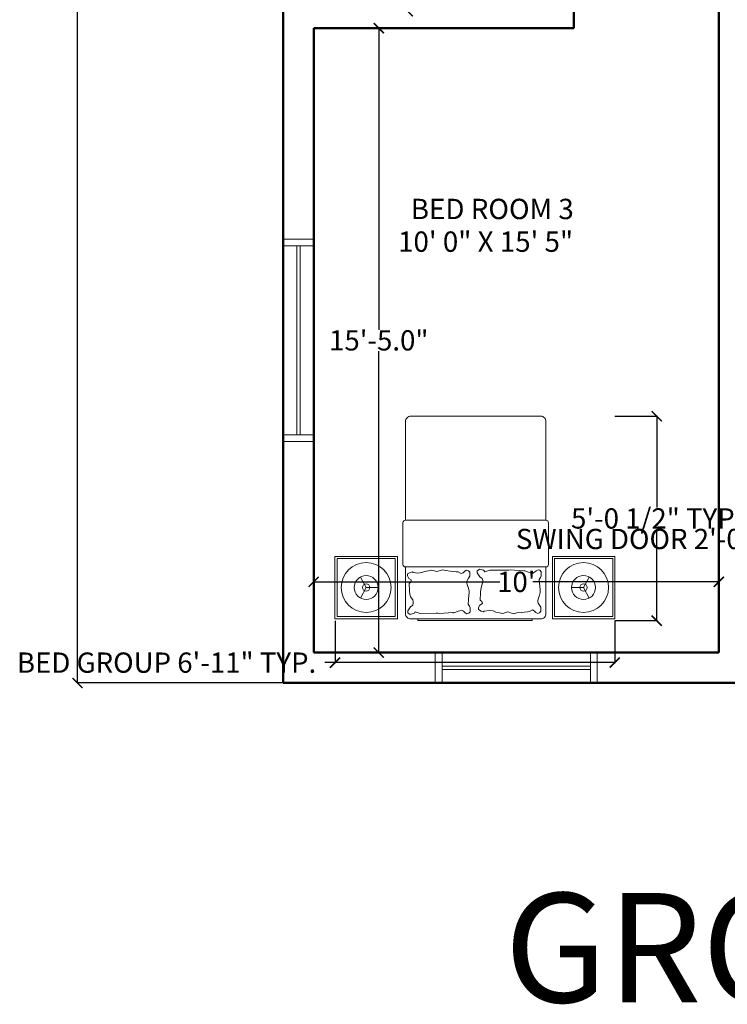
# Model space of a CAD drawing. Units: inches. Extents: x 147 to 1638, y 107 to 941.
# Tile 1 of 17: x 147 to 356, y 107 to 398. Entities that reach past the tile are written whole.
import ezdxf

# ---------------------------------------------------------------- set-up
doc = ezdxf.new("R2010")
doc.units = ezdxf.units.IN
doc.header["$MEASUREMENT"] = 0
for name, color, linetype, lineweight in [('A-ANNO-DIMS', 2, 'Continuous', 15), ('A-ANNO-TEXT', 7, 'Continuous', 25), ('A-AREA-IDEN', 7, 'Continuous', 18), ('furniture', 50, 'Continuous', 18), ('walls', 7, 'Continuous', 50), ('windows', 3, 'Continuous', 20)]:
    doc.layers.add(name, color=color, linetype=linetype, lineweight=lineweight)
doc.styles.get("Standard").update_dxf_attribs({"font": 'arial.ttf'})
doc.dimstyles.get("Standard").update_dxf_attribs({"dimtxt": 6, "dimasz": 3, "dimexe": 0.18, "dimexo": 0.0625, "dimgap": 0.09, "dimtad": 0, "dimtih": 1, "dimtoh": 1, "dimdec": 1, "dimzin": 0, "dimdsep": 46, "dimlunit": 3, "dimtxsty": 'Standard', "dimblk": 'ARCHTICK', "dimcen": 0.09, "dimadec": 0, "dimazin": 0, "dimtfac": 1, "dimtdec": 1, "dimtofl": 0, "dimtmove": 0, "dimatfit": 3, "dimfxl": 1, "dimtolj": 1, "dimtzin": 0, "dimarcsym": 0})

# ---------------------------------------------------------------- blocks, each defined once
blk = doc.blocks.new('_ArchTick')
at = {"color": 0, "linetype": 'ByBlock', "const_width": 0.15}
blk.add_lwpolyline([(-0.5, -0.5), (0.5, 0.5)], dxfattribs=at)
blk = doc.blocks.new('*D24')
at = {"layer": 'A-ANNO-DIMS', "color": 0, "lineweight": -2, "transparency": 16777216}
for p, q in [((248.22, 395.72), (253.39, 395.72)), ((253.21, 395.72), (253.21, 306.37)), ((253.21, 210.72), (253.21, 300.06)), ((248.22, 210.72), (253.39, 210.72))]:
    blk.add_line(p, q, dxfattribs=at)
at = {"layer": 'Defpoints', "color": 0, "lineweight": -2, "transparency": 16777216}
for p in [(248.16, 395.72), (248.16, 210.72), (253.21, 210.72)]:
    blk.add_point(p, dxfattribs=at)
at = {"layer": 'A-ANNO-DIMS', "color": 0, "lineweight": -2, "transparency": 16777216, "xscale": 3, "yscale": 3, "zscale": 3}
for p, rotation in [((253.21, 395.72), 90), ((253.21, 210.72), 270)]:
    blk.add_blockref('_ArchTick', p, dxfattribs=dict(at, rotation=rotation))
at = {"layer": 'A-ANNO-DIMS', "color": 0, "transparency": 16777216, "insert": (253.21, 303.22), "char_height": 6, "attachment_point": 5}
blk.add_mtext('\\A1;15\'-5.0"', dxfattribs=at)
blk = doc.blocks.new('*D25')
at = {"layer": 'A-ANNO-DIMS', "color": 0, "lineweight": -2, "transparency": 16777216}
for p, q in [((233.94, 245.59), (233.94, 231.49)), ((353.94, 245.59), (353.94, 231.49)), ((233.94, 231.67), (289.05, 231.67)), ((353.94, 231.67), (298.84, 231.67))]:
    blk.add_line(p, q, dxfattribs=at)
at = {"layer": 'Defpoints', "color": 0, "lineweight": -2, "transparency": 16777216}
for p in [(233.94, 245.65), (353.94, 245.65), (353.94, 231.67)]:
    blk.add_point(p, dxfattribs=at)
at = {"layer": 'A-ANNO-DIMS', "color": 0, "lineweight": -2, "transparency": 16777216, "xscale": 3, "yscale": 3, "zscale": 3, "rotation": 180}
blk.add_blockref('_ArchTick', (233.94, 231.67), dxfattribs=at)
at = {"layer": 'A-ANNO-DIMS', "color": 0, "lineweight": -2, "transparency": 16777216, "xscale": 3, "yscale": 3, "zscale": 3}
blk.add_blockref('_ArchTick', (353.94, 231.67), dxfattribs=at)
at = {"layer": 'A-ANNO-DIMS', "color": 0, "transparency": 16777216, "insert": (293.94, 231.67), "char_height": 6, "attachment_point": 5}
blk.add_mtext("\\A1;10'", dxfattribs=at)
blk = doc.blocks.new('*D70')
at = {"layer": 'A-ANNO-DIMS', "color": 0, "lineweight": -2, "transparency": 16777216}
for p, q in [((224.88, 909.72), (163.8, 909.72)), ((163.98, 909.72), (163.98, 558.87)), ((163.98, 201.72), (163.98, 552.56)), ((224.88, 201.72), (163.8, 201.72))]:
    blk.add_line(p, q, dxfattribs=at)
at = {"layer": 'Defpoints', "color": 0, "lineweight": -2, "transparency": 16777216}
for p in [(224.94, 909.72), (163.98, 201.72), (224.94, 201.72)]:
    blk.add_point(p, dxfattribs=at)
at = {"layer": 'A-ANNO-DIMS', "color": 0, "lineweight": -2, "transparency": 16777216, "xscale": 3, "yscale": 3, "zscale": 3}
for p, rotation in [((163.98, 909.72), 90), ((163.98, 201.72), 270)]:
    blk.add_blockref('_ArchTick', p, dxfattribs=dict(at, rotation=rotation))
at = {"layer": 'A-ANNO-DIMS', "color": 0, "transparency": 16777216, "insert": (163.98, 555.72), "char_height": 6, "attachment_point": 5}
blk.add_mtext("\\A1;59'", dxfattribs=at)
blk = doc.blocks.new('MAT-P14')
for p, q in [((-1.3369, 1.348), (-1.3369, 1.948)), ((-1.3369, 1.948), (-0.7369, 1.948)), ((-1.3169, 1.928), (-0.7569, 1.928)), ((-1.3169, 1.368), (-1.3169, 1.928)), ((-0.7569, 1.368), (-0.7569, 1.928)), ((-0.7369, 1.348), (-0.7369, 1.948)), ((0.625, 1.95), (-0.625, 1.95)), ((0.7534, 1.348), (0.7534, 1.948)), ((1.3534, 1.948), (0.7534, 1.948)), ((1.3334, 1.928), (0.7734, 1.928)), ((0.7734, 1.368), (0.7734, 1.928)), ((1.3334, 1.368), (1.3334, 1.928)), ((1.3534, 1.348), (1.3534, 1.948)), ((-1.0369, 1.648), (-1.0913, 1.7493)), ((1.0534, 1.648), (1.1078, 1.7493)), ((-1.0369, 1.648), (-1.0913, 1.5467)), ((-1.0369, 1.648), (-0.9219, 1.648)), ((1.0534, 1.648), (0.9384, 1.648)), ((1.0534, 1.648), (1.1078, 1.5467)), ((-1.3369, 1.348), (-0.7369, 1.348)), ((-1.3169, 1.368), (-0.7569, 1.368)), ((1.3534, 1.348), (0.7534, 1.348)), ((1.3334, 1.368), (0.7734, 1.368))]:
    blk.add_line(p, q)
for points in [[(-0.675, 1.45), (-0.675, 1.9, -0.414214), (-0.625, 1.95), (0.625, 1.95, -0.414214), (0.675, 1.9), (0.675, 1.45)], [(-0.675, 1, -0.414214), (-0.7, 1.025), (-0.7, 1.425, -0.414214), (-0.675, 1.45), (0.675, 1.45, -0.414214), (0.7, 1.425), (0.7, 1.025, -0.414214), (0.675, 1)], [(-0.625, 0, -0.414214), (-0.675, 0.05), (-0.675, 1), (0.675, 1), (0.675, 0.05, -0.414214), (0.625, 0)]]:
    blk.add_lwpolyline(points, format="xyb", close=True)
for points in [[(-0.6142, 1.8182), (-0.6262, 1.8377), (-0.6262, 1.8767), (-0.6142, 1.8914), (-0.5964, 1.8963), (-0.5785, 1.8865), (-0.563, 1.8719), (-0.5451, 1.8633), (-0.5157, 1.879), (-0.4966, 1.8816), (-0.4647, 1.8842), (-0.4393, 1.8868), (-0.3947, 1.892), (-0.3629, 1.8999), (-0.3094, 1.8823), (-0.2619, 1.8969), (-0.23, 1.8916), (-0.1918, 1.8838), (-0.1664, 1.8734), (-0.1282, 1.8682), (-0.0818, 1.8753), (-0.0758, 1.8802), (-0.052, 1.8753), (-0.0281, 1.8607), (-0.0281, 1.8412), (-0.0401, 1.8168), (-0.0639, 1.8022), (-0.0598, 1.781), (-0.0431, 1.7682), (-0.0463, 1.6973), (-0.0502, 1.6621), (-0.0561, 1.6397), (-0.0619, 1.6125), (-0.0678, 1.5965), (-0.0678, 1.5789), (-0.0631, 1.5599), (-0.0393, 1.5453), (-0.0147, 1.5053), (-0.0147, 1.4858), (-0.0385, 1.4711), (-0.0751, 1.4819), (-0.081, 1.4868), (-0.087, 1.4965), (-0.1344, 1.4812), (-0.3042, 1.4815), (-0.3178, 1.4815), (-0.3355, 1.4791), (-0.4636, 1.4878), (-0.4672, 1.4865), (-0.4732, 1.4863), (-0.5167, 1.5026), (-0.5299, 1.5053), (-0.5478, 1.5102), (-0.5656, 1.5015), (-0.5812, 1.4869), (-0.599, 1.4772), (-0.6169, 1.482), (-0.6288, 1.4967), (-0.6288, 1.5357), (-0.6229, 1.5503), (-0.611, 1.5698), (-0.6136, 1.6138), (-0.6149, 1.6269), (-0.6176, 1.6443), (-0.6189, 1.6595), (-0.6202, 1.6748), (-0.6202, 1.6955), (-0.6176, 1.7075), (-0.6136, 1.7227), (-0.6083, 1.7391), (-0.6043, 1.75), (-0.5976, 1.7707), (-0.5963, 1.7848), (-0.6003, 1.7979), (-0.6136, 1.8186)], [(0.0694, 1.5591), (0.0575, 1.5396), (0.0575, 1.5006), (0.0694, 1.4859), (0.0873, 1.481), (0.1052, 1.4908), (0.1207, 1.5054), (0.1386, 1.514), (0.168, 1.4983), (0.1871, 1.4957), (0.2189, 1.4931), (0.2444, 1.4905), (0.289, 1.4853), (0.3208, 1.4774), (0.3742, 1.495), (0.4218, 1.4804), (0.4536, 1.4857), (0.4918, 1.4935), (0.5173, 1.5039), (0.5555, 1.5091), (0.6019, 1.502), (0.6079, 1.4971), (0.6317, 1.502), (0.6555, 1.5166), (0.6555, 1.5361), (0.6436, 1.5605), (0.6198, 1.5751), (0.6239, 1.5963), (0.6405, 1.6091), (0.6373, 1.68), (0.6334, 1.7152), (0.6276, 1.7376), (0.6063, 1.7648), (0.6005, 1.7808), (0.6005, 1.7984), (0.6051, 1.8174), (0.6289, 1.832), (0.6536, 1.872), (0.6536, 1.8915), (0.6298, 1.9062), (0.5932, 1.8954), (0.5872, 1.8905), (0.5813, 1.8808), (0.5338, 1.8961), (0.3795, 1.8958), (0.3658, 1.8958), (0.3482, 1.8982), (0.2201, 1.8895), (0.2165, 1.8908), (0.2104, 1.891), (0.1669, 1.8747), (0.1538, 1.872), (0.1359, 1.8671), (0.118, 1.8758), (0.1025, 1.8904), (0.0846, 1.9001), (0.0667, 1.8953), (0.0548, 1.8806), (0.0548, 1.8416), (0.0608, 1.827), (0.0727, 1.8075), (0.0701, 1.7635), (0.0688, 1.7504), (0.0661, 1.733), (0.0648, 1.7178), (0.0634, 1.7025), (0.0634, 1.6818), (0.0661, 1.6698), (0.0701, 1.6546), (0.0754, 1.6382), (0.0794, 1.6273), (0.086, 1.6066), (0.0874, 1.5925), (0.0834, 1.5794), (0.0701, 1.5587)]]:
    blk.add_lwpolyline(points)
blk.add_lwpolyline([(-0.5417, 1.95), (-0.5417, 1.9665), (0.5583, 1.9665), (0.5583, 1.95)], close=True)
for centre, radius in [((-1.0369, 1.648), 0.24), ((1.0534, 1.648), 0.24), ((-1.0369, 1.648), 0.115), ((1.0534, 1.648), 0.115), ((-1.0369, 1.648), 0.035), ((1.0534, 1.648), 0.035)]:
    blk.add_circle(centre, radius)
blk = doc.blocks.new('WIN-60IN')
for p, q in [((60, 9), (0, 9)), ((0, 9), (0, 0)), ((2, 9), (2, 0)), ((58, 0), (58, 9)), ((60, 0), (60, 9)), ((2, 5), (58, 5)), ((2, 4), (58, 4)), ((0, 0), (60, 0))]:
    blk.add_line(p, q)
blk = doc.blocks.new('WIN-48IN')
for p, q in [((9, 48), (0, 48)), ((0, 48), (0, 0)), ((9, 0), (9, 48)), ((9, 46), (0, 46)), ((4, 2), (4, 46)), ((5, 2), (5, 46)), ((0, 2), (9, 2)), ((0, 0), (9, 0))]:
    blk.add_line(p, q)
blk = doc.blocks.new('*D98')
at = {"layer": 'A-ANNO-DIMS', "color": 0, "lineweight": -2, "transparency": 16777216}
for p, q in [((388.94, 247.92), (388.94, 244.2)), ((412.94, 247.92), (412.94, 244.2)), ((388.94, 244.38), (385.94, 244.38)), ((412.94, 244.38), (388.94, 244.38))]:
    blk.add_line(p, q, dxfattribs=at)
at = {"layer": 'Defpoints', "color": 0, "lineweight": -2, "transparency": 16777216}
for p in [(388.94, 247.98), (412.94, 247.98), (388.94, 244.38)]:
    blk.add_point(p, dxfattribs=at)
at = {"layer": 'A-ANNO-DIMS', "color": 0, "lineweight": -2, "transparency": 16777216, "xscale": 3, "yscale": 3, "zscale": 3, "rotation": 180}
blk.add_blockref('_ArchTick', (388.94, 244.38), dxfattribs=at)
at = {"layer": 'A-ANNO-DIMS', "color": 0, "lineweight": -2, "transparency": 16777216, "xscale": 3, "yscale": 3, "zscale": 3}
blk.add_blockref('_ArchTick', (412.94, 244.38), dxfattribs=at)
at = {"layer": 'A-ANNO-DIMS', "color": 0, "transparency": 16777216, "insert": (338.48, 244.38), "char_height": 6, "attachment_point": 5}
blk.add_mtext('\\A1;SWING DOOR 2\'-0" TYP.', dxfattribs=at)
blk = doc.blocks.new('*D110')
at = {"layer": 'A-ANNO-DIMS', "color": 0, "lineweight": -2, "transparency": 16777216}
for p, q in [((240.25, 220.12), (240.25, 207.57)), ((323.11, 220.12), (323.11, 207.57)), ((240.25, 207.75), (237.25, 207.75)), ((323.11, 207.75), (240.25, 207.75))]:
    blk.add_line(p, q, dxfattribs=at)
at = {"layer": 'Defpoints', "color": 0, "lineweight": -2, "transparency": 16777216}
for p in [(240.25, 220.18), (323.11, 220.18), (240.25, 207.75)]:
    blk.add_point(p, dxfattribs=at)
at = {"layer": 'A-ANNO-DIMS', "color": 0, "lineweight": -2, "transparency": 16777216, "xscale": 3, "yscale": 3, "zscale": 3, "rotation": 180}
blk.add_blockref('_ArchTick', (240.25, 207.75), dxfattribs=at)
at = {"layer": 'A-ANNO-DIMS', "color": 0, "lineweight": -2, "transparency": 16777216, "xscale": 3, "yscale": 3, "zscale": 3}
blk.add_blockref('_ArchTick', (323.11, 207.75), dxfattribs=at)
at = {"layer": 'A-ANNO-DIMS', "color": 0, "transparency": 16777216, "insert": (190.36, 207.75), "char_height": 6, "attachment_point": 5}
blk.add_mtext('\\A1;BED GROUP 6\'-11" TYP.', dxfattribs=at)
blk = doc.blocks.new('*D111')
at = {"layer": 'A-ANNO-DIMS', "color": 0, "lineweight": -2, "transparency": 16777216}
for p, q in [((323.17, 280.75), (335.72, 280.75)), ((335.54, 280.75), (335.54, 253.66)), ((335.54, 220.18), (335.54, 247.27)), ((323.17, 220.18), (335.72, 220.18))]:
    blk.add_line(p, q, dxfattribs=at)
at = {"layer": 'Defpoints', "color": 0, "lineweight": -2, "transparency": 16777216}
for p in [(323.11, 280.75), (323.11, 220.18), (335.54, 220.18)]:
    blk.add_point(p, dxfattribs=at)
at = {"layer": 'A-ANNO-DIMS', "color": 0, "lineweight": -2, "transparency": 16777216, "xscale": 3, "yscale": 3, "zscale": 3}
for p, rotation in [((335.54, 280.75), 90), ((335.54, 220.18), 270)]:
    blk.add_blockref('_ArchTick', p, dxfattribs=dict(at, rotation=rotation))
at = {"layer": 'A-ANNO-DIMS', "color": 0, "transparency": 16777216, "insert": (335.54, 250.46), "char_height": 6, "attachment_point": 5}
blk.add_mtext('\\A1;5\'-0 1/2" TYP.', dxfattribs=at)
blk = doc.blocks.new('*D120')
at = {"layer": 'A-ANNO-DIMS', "color": 0, "lineweight": -2, "transparency": 16777216}
for p, q in [((263.65, 412.63), (260.65, 412.63)), ((263.65, 410.81), (263.65, 412.81)), ((276.23, 412.63), (263.65, 412.63)), ((276.23, 410.81), (276.23, 412.81))]:
    blk.add_line(p, q, dxfattribs=at)
at = {"layer": 'Defpoints', "color": 0, "lineweight": -2, "transparency": 16777216}
for p in [(263.65, 412.63), (263.65, 410.74), (276.23, 410.74)]:
    blk.add_point(p, dxfattribs=at)
at = {"layer": 'A-ANNO-DIMS', "color": 0, "lineweight": -2, "transparency": 16777216, "xscale": 3, "yscale": 3, "zscale": 3, "rotation": 180}
blk.add_blockref('_ArchTick', (263.65, 412.63), dxfattribs=at)
at = {"layer": 'A-ANNO-DIMS', "color": 0, "lineweight": -2, "transparency": 16777216, "xscale": 3, "yscale": 3, "zscale": 3}
blk.add_blockref('_ArchTick', (276.23, 412.63), dxfattribs=at)
at = {"layer": 'A-ANNO-DIMS', "color": 0, "transparency": 16777216, "insert": (221.68, 412.63), "char_height": 6, "attachment_point": 5}
blk.add_mtext('\\A1;BASIN 1\'-0 1/2" TYP.', dxfattribs=at)
blk = doc.blocks.new('*D121')
at = {"layer": 'A-ANNO-DIMS', "color": 0, "lineweight": -2, "transparency": 16777216}
for p, q in [((263.59, 410.74), (261.59, 410.74)), ((261.77, 410.74), (261.77, 408.88)), ((261.77, 400.72), (261.77, 402.58)), ((263.59, 400.72), (261.59, 400.72))]:
    blk.add_line(p, q, dxfattribs=at)
at = {"layer": 'Defpoints', "color": 0, "lineweight": -2, "transparency": 16777216}
for p in [(263.65, 410.74), (261.77, 400.72), (263.65, 400.72)]:
    blk.add_point(p, dxfattribs=at)
at = {"layer": 'A-ANNO-DIMS', "color": 0, "lineweight": -2, "transparency": 16777216, "xscale": 3, "yscale": 3, "zscale": 3}
for p, rotation in [((261.77, 410.74), 90), ((261.77, 400.72), 270)]:
    blk.add_blockref('_ArchTick', p, dxfattribs=dict(at, rotation=rotation))
at = {"layer": 'A-ANNO-DIMS', "color": 0, "transparency": 16777216, "insert": (261.77, 405.73), "char_height": 6, "attachment_point": 5}
blk.add_mtext('\\A1;0\'-10" TYP.', dxfattribs=at)

msp = doc.modelspace()

# ---------------------------------------------------------------- linework, layer by layer
at = {"layer": 'walls'}
for p, q in [((224.94, 909.72), (224.94, 201.72)), ((310.94, 448.72), (310.94, 395.72)), ((353.94, 436.72), (353.94, 210.72)), ((233.94, 395.72), (310.94, 395.72)), ((233.94, 395.72), (233.94, 210.72)), ((233.94, 210.72), (353.94, 210.72)), ((224.94, 201.72), (358.94, 201.72))]:
    msp.add_line(p, q, dxfattribs=at)

# ---------------------------------------------------------------- block references
at = {"layer": 'furniture', "xscale": 30.80045642108221, "yscale": 30.80045642108221, "zscale": 30.80045642108221, "rotation": 180}
msp.add_blockref('MAT-P14', (281.93, 280.75), dxfattribs=at)
at = {"layer": 'windows'}
for name, p, rotation in [('WIN-60IN', (224.94, 333.22), 270.0000000000006), ('WIN-48IN', (269.94, 210.72), 270.0000000000001)]:
    msp.add_blockref(name, p, dxfattribs=dict(at, rotation=rotation))

# ---------------------------------------------------------------- texts
at = {"layer": 'A-ANNO-TEXT'}
msp.add_text('GROUND FLOOR', height=32.387, dxfattribs=at).set_placement((290.4, 107.1))
at = {"layer": 'A-AREA-IDEN'}
for s, height, p in [('BED ROOM 3', 6.031, (262.69, 339.13)), ('  10\' 0" X 15\' 5"', 6.0306, (255.24, 329.45))]:
    msp.add_text(s, height=height, dxfattribs=at).set_placement(p)

# ---------------------------------------------------------------- dimensions: what is measured, and where the dimension line sits
at = {"layer": 'A-ANNO-DIMS'}
for base, p1, p2, picture, middle in [((163.98, 201.72), (224.94, 909.72), (224.94, 201.72), '*D70', (163.98, 555.72)), ((253.21, 210.72), (248.16, 395.72), (248.16, 210.72), '*D24', (253.21, 303.22))]:
    dim = msp.add_linear_dim(base=base, p1=p1, p2=p2, angle=90, dimstyle='Standard', override={"dimclrd": 0, "dimclre": 0, "dimclrt": 0}, dxfattribs=at)
    dim.commit()
    dim.dimension.update_dxf_attribs({"geometry": picture, "text_midpoint": middle})
for base, p1, p2, angle, text, picture, middle in [((263.65, 412.63), (276.23, 410.74), (263.65, 410.74), 180, 'BASIN <> TYP.', '*D120', (221.68, 412.63)), ((261.77, 400.72), (263.65, 410.74), (263.65, 400.72), 270, '<> TYP.', '*D121', (261.77, 405.73)), ((335.54, 220.18), (323.11, 280.75), (323.11, 220.18), 270, '<> TYP.', '*D111', (335.54, 250.46)), ((388.94, 244.38), (412.94, 247.98), (388.94, 247.98), 180, 'SWING DOOR <> TYP.', '*D98', (338.48, 244.38)), ((240.25, 207.75), (323.11, 220.18), (240.25, 220.18), 180, 'BED GROUP <> TYP.', '*D110', (190.36, 207.75))]:
    dim = msp.add_linear_dim(base=base, p1=p1, p2=p2, angle=angle, text=text, dimstyle='Standard', override={"dimdec": 1, "dimlfac": 1, "dimrnd": 0, "dimzin": 1, "dimdsep": 46, "dimlunit": 4, "dimfrac": 2}, dxfattribs=at)
    dim.commit()
    dim.dimension.update_dxf_attribs({"geometry": picture, "text_midpoint": middle})
dim = msp.add_linear_dim(base=(353.94, 231.67), p1=(233.94, 245.65), p2=(353.94, 245.65), dimstyle='Standard', override={"dimclrd": 0, "dimclre": 0, "dimclrt": 0}, dxfattribs=at)
dim.commit()
dim.dimension.update_dxf_attribs({"geometry": '*D25', "text_midpoint": (293.94, 231.67)})

doc.saveas('drawing.dxf')
